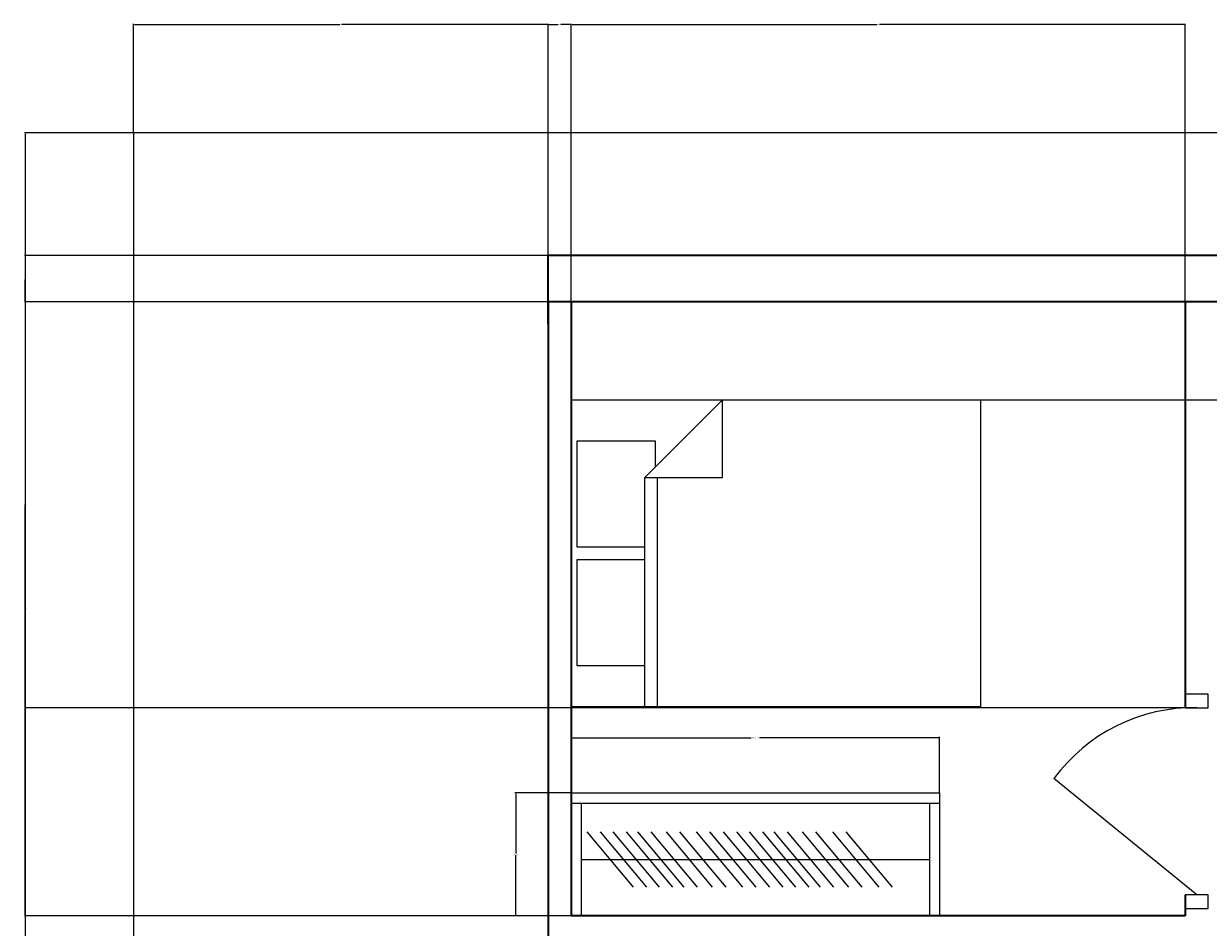
# Model space of a CAD drawing. Units: inches. Extents: x 109 to 572, y -157 to 568.
# Tile 2 of 5: x 109 to 341, y 391 to 568. Entities that reach past the tile are written whole.
import ezdxf

# ---------------------------------------------------------------- set-up
doc = ezdxf.new("R2010")
doc.units = ezdxf.units.IN
for name, color, linetype, lineweight in [('A-ANNO-DIMS', 2, 'Continuous', 18), ('A-FLOR-CASE', 32, 'Continuous', 18), ('A-WALL', 7, 'Continuous', 35), ('C-PROP', 8, 'Continuous', 18), ('DOOR.', 240, 'Continuous', 25), ('FURNUTURE', 50, 'Continuous', 18)]:
    doc.layers.add(name, color=color, linetype=linetype, lineweight=lineweight)
doc.styles.get("Standard").update_dxf_attribs({"font": 'arial.ttf'})
doc.dimstyles.get("Standard").update_dxf_attribs({"dimtxt": 0.18, "dimasz": 0.18, "dimexe": 0.18, "dimexo": 0.0625, "dimgap": 0.09, "dimtad": 0, "dimtih": 1, "dimtoh": 1, "dimdec": 4, "dimzin": 0, "dimdsep": 46, "dimtxsty": 'Standard', "dimcen": 0.09, "dimadec": 0, "dimazin": 0, "dimtfac": 1, "dimtdec": 4, "dimtofl": 0, "dimtmove": 0, "dimatfit": 3, "dimfxl": 1, "dimtolj": 1, "dimtzin": 0, "dimarcsym": 0})

# ---------------------------------------------------------------- blocks, each defined once
blk = doc.blocks.new('Bed - Queen')
for p, q in [((0, -80.00003), (0, 0)), ((0, 0), (59.99999, 0)), ((59.99999, 0), (59.99999, -80.00003)), ((7.99999, -1.2), (28.79998, -1.2)), ((7.99999, -14.4), (7.99999, -1.2)), ((28.79998, -1.2), (28.79998, -14.4)), ((31.19999, -1.2), (51.99999, -1.2)), ((31.19999, -14.4), (31.19999, -1.2)), ((51.99999, -1.2), (51.99999, -16.4)), ((0, -14.4), (44.8, -14.4)), ((59.99999, -29.6), (44.8, -14.4)), ((44.8, -14.4), (44.8, -29.6)), ((44.8, -16.8), (0, -16.8)), ((51.99999, -16.4), (46.79936, -16.4)), ((44.8, -29.6), (59.99999, -29.6)), ((59.99999, -80.00003), (0, -80.00003))]:
    blk.add_line(p, q)
blk = doc.blocks.new('DOOR-SINGLE-36IN-JAMB')
blk.add_line((0, 0), (-27.91, 22.73))
for points in [[(-2.25, 36.57), (2.25, 36.57), (2.25, 39.21), (-2.25, 39.21)], [(-2.25, -2.64), (2.25, -2.64), (2.25, 0), (-2.25, 0)]]:
    blk.add_lwpolyline(points, close=True)
blk.add_arc((-0.58, 2.67), 33.9, 89.0125, 143.7179)
blk = doc.blocks.new('CLOSET-FRAME-RAIL-72IN')
for p, q in [((0, 0), (0, 24)), ((0, 24), (72, 24)), ((72, 24), (72, 0)), ((0, 22), (72, 22)), ((2, 0), (2, 22)), ((70, 22), (70, 0)), ((2, 11), (70, 11))]:
    blk.add_line(p, q)
blk = doc.blocks.new('CLOSET-HANGERS')
for p, q in [((0, 0), (-9.05, 10.83)), ((2.61, -0.01), (-6.44, 10.82)), ((5.08, -0.01), (-3.97, 10.82)), ((7.69, -0.01), (-1.36, 10.82)), ((9.9, -0.01), (0.85, 10.82)), ((12.51, -0.01), (3.46, 10.82)), ((15.48, -0.01), (6.43, 10.82)), ((18.09, -0.01), (9.04, 10.82)), ((21.4, -0.01), (12.35, 10.82)), ((24.01, -0.01), (14.96, 10.82)), ((26.62, 0.01), (17.57, 10.84)), ((29.23, 0), (20.18, 10.83)), ((31.7, 0), (22.65, 10.83)), ((34.31, -0.01), (25.26, 10.82)), ((36.52, 0), (27.47, 10.83)), ((39.13, -0.01), (30.08, 10.82)), ((42.1, 0), (33.05, 10.83)), ((44.71, -0.01), (35.66, 10.82)), ((48.01, 0), (38.97, 10.83)), ((50.63, -0.01), (41.58, 10.82))]:
    blk.add_line(p, q)
blk = doc.blocks.new('*D25')
at = {"layer": 'A-ANNO-DIMS', "color": 0, "lineweight": -2, "transparency": 16777216}
for p, q in [((216.02, 417.6), (216.02, 428.52)), ((216.2, 428.34), (251.18, 428.34)), ((287.84, 428.34), (252.86, 428.34)), ((288.02, 417.6), (288.02, 428.52))]:
    blk.add_line(p, q, dxfattribs=at)
at = {"layer": 'A-ANNO-DIMS', "color": 0, "transparency": 16777216}
for points in [[(216.2, 428.37), (216.2, 428.31), (216.02, 428.34)], [(287.84, 428.37), (287.84, 428.31), (288.02, 428.34)]]:
    blk.add_solid(points, dxfattribs=at)
at = {"layer": 'Defpoints', "color": 0, "transparency": 16777216}
for p in [(288.02, 428.34), (216.02, 417.54), (288.02, 417.54)]:
    blk.add_point(p, dxfattribs=at)
at = {"layer": 'A-ANNO-DIMS', "color": 0, "transparency": 16777216, "insert": (252.02, 428.34), "char_height": 0.18, "attachment_point": 5}
blk.add_mtext('\\A1;RAIL 72 TYP.', dxfattribs=at)
blk = doc.blocks.new('*D26')
at = {"layer": 'A-ANNO-DIMS', "color": 0, "lineweight": -2, "transparency": 16777216}
for p, q in [((215.96, 417.54), (205.04, 417.54)), ((205.22, 417.36), (205.22, 405.72)), ((205.22, 393.72), (205.22, 405.36)), ((215.96, 393.54), (205.04, 393.54))]:
    blk.add_line(p, q, dxfattribs=at)
at = {"layer": 'A-ANNO-DIMS', "color": 0, "transparency": 16777216}
for points in [[(205.19, 417.36), (205.25, 417.36), (205.22, 417.54)], [(205.19, 393.72), (205.25, 393.72), (205.22, 393.54)]]:
    blk.add_solid(points, dxfattribs=at)
at = {"layer": 'Defpoints', "color": 0, "transparency": 16777216}
for p in [(205.22, 417.54), (216.02, 417.54), (216.02, 393.54)]:
    blk.add_point(p, dxfattribs=at)
at = {"layer": 'A-ANNO-DIMS', "color": 0, "transparency": 16777216, "insert": (205.22, 405.54), "char_height": 0.18, "attachment_point": 5}
blk.add_mtext('\\A1;24 TYP.', dxfattribs=at)
blk = doc.blocks.new('*D40')
at = {"layer": 'A-ANNO-DIMS', "color": 0, "lineweight": -2, "transparency": 16777216}
for p, q in [((130.46, 546.54), (109.19, 546.54)), ((109.37, 546.36), (109.37, 336.72)), ((109.37, 126.72), (109.37, 336.36)), ((130.46, 126.54), (109.19, 126.54))]:
    blk.add_line(p, q, dxfattribs=at)
at = {"layer": 'A-ANNO-DIMS', "color": 0, "transparency": 16777216}
for points in [[(109.34, 546.36), (109.4, 546.36), (109.37, 546.54)], [(109.34, 126.72), (109.4, 126.72), (109.37, 126.54)]]:
    blk.add_solid(points, dxfattribs=at)
at = {"layer": 'Defpoints', "color": 0, "transparency": 16777216}
for p in [(109.37, 546.54), (130.52, 546.54), (130.52, 126.54)]:
    blk.add_point(p, dxfattribs=at)
at = {"layer": 'A-ANNO-DIMS', "color": 0, "transparency": 16777216, "insert": (109.37, 336.54), "char_height": 0.18, "attachment_point": 5}
blk.add_mtext('\\A1;420', dxfattribs=at)
blk = doc.blocks.new('*D41')
at = {"layer": 'A-ANNO-DIMS', "color": 0, "lineweight": -2, "transparency": 16777216}
for p, q in [((130.52, 546.6), (130.52, 567.87)), ((130.7, 567.69), (170.82, 567.69)), ((211.34, 567.69), (171.22, 567.69)), ((211.52, 522.6), (211.52, 567.87))]:
    blk.add_line(p, q, dxfattribs=at)
at = {"layer": 'A-ANNO-DIMS', "color": 0, "transparency": 16777216}
for points in [[(130.7, 567.72), (130.7, 567.66), (130.52, 567.69)], [(211.34, 567.72), (211.34, 567.66), (211.52, 567.69)]]:
    blk.add_solid(points, dxfattribs=at)
at = {"layer": 'Defpoints', "color": 0, "transparency": 16777216}
for p in [(211.52, 567.69), (130.52, 546.54), (211.52, 522.54)]:
    blk.add_point(p, dxfattribs=at)
at = {"layer": 'A-ANNO-DIMS', "color": 0, "transparency": 16777216, "insert": (171.02, 567.69), "char_height": 0.18, "attachment_point": 5}
blk.add_mtext('\\A1;81', dxfattribs=at)
blk = doc.blocks.new('*D45')
at = {"layer": 'A-ANNO-DIMS', "color": 0, "lineweight": -2, "transparency": 16777216}
for p, q in [((216.02, 513.6), (216.02, 567.87)), ((216.2, 567.69), (275.74, 567.69)), ((335.84, 567.69), (276.3, 567.69)), ((336.02, 513.6), (336.02, 567.87))]:
    blk.add_line(p, q, dxfattribs=at)
at = {"layer": 'A-ANNO-DIMS', "color": 0, "transparency": 16777216}
for points in [[(216.2, 567.72), (216.2, 567.66), (216.02, 567.69)], [(335.84, 567.72), (335.84, 567.66), (336.02, 567.69)]]:
    blk.add_solid(points, dxfattribs=at)
at = {"layer": 'Defpoints', "color": 0, "transparency": 16777216}
for p in [(336.02, 567.69), (216.02, 513.54), (336.02, 513.54)]:
    blk.add_point(p, dxfattribs=at)
at = {"layer": 'A-ANNO-DIMS', "color": 0, "transparency": 16777216, "insert": (276.02, 567.69), "char_height": 0.18, "attachment_point": 5}
blk.add_mtext('\\A1;120', dxfattribs=at)
blk = doc.blocks.new('*D50')
at = {"layer": 'A-ANNO-DIMS', "color": 0, "lineweight": -2, "transparency": 16777216}
for p, q in [((215.96, 513.54), (109.19, 513.54)), ((109.37, 513.36), (109.37, 453.72)), ((109.37, 393.72), (109.37, 453.36)), ((215.96, 393.54), (109.19, 393.54))]:
    blk.add_line(p, q, dxfattribs=at)
at = {"layer": 'A-ANNO-DIMS', "color": 0, "transparency": 16777216}
for points in [[(109.34, 513.36), (109.4, 513.36), (109.37, 513.54)], [(109.34, 393.72), (109.4, 393.72), (109.37, 393.54)]]:
    blk.add_solid(points, dxfattribs=at)
at = {"layer": 'Defpoints', "color": 0, "transparency": 16777216}
for p in [(109.37, 513.54), (216.02, 513.54), (216.02, 393.54)]:
    blk.add_point(p, dxfattribs=at)
at = {"layer": 'A-ANNO-DIMS', "color": 0, "transparency": 16777216, "insert": (109.37, 453.54), "char_height": 0.18, "attachment_point": 5}
blk.add_mtext('\\A1;120', dxfattribs=at)
blk = doc.blocks.new('*D57')
at = {"layer": 'A-ANNO-DIMS', "color": 0, "lineweight": -2, "transparency": 16777216}
for p, q in [((335.96, 513.54), (109.19, 513.54)), ((109.37, 513.36), (109.37, 474.05)), ((109.37, 434.39), (109.37, 473.69)), ((335.96, 434.21), (109.19, 434.21))]:
    blk.add_line(p, q, dxfattribs=at)
at = {"layer": 'A-ANNO-DIMS', "color": 0, "transparency": 16777216}
for points in [[(109.34, 513.36), (109.4, 513.36), (109.37, 513.54)], [(109.34, 434.39), (109.4, 434.39), (109.37, 434.21)]]:
    blk.add_solid(points, dxfattribs=at)
at = {"layer": 'Defpoints', "color": 0, "transparency": 16777216}
for p in [(336.02, 513.54), (109.37, 434.21), (336.02, 434.21)]:
    blk.add_point(p, dxfattribs=at)
at = {"layer": 'A-ANNO-DIMS', "color": 0, "transparency": 16777216, "insert": (109.37, 473.87), "char_height": 0.18, "attachment_point": 5}
blk.add_mtext('\\A1;79.33', dxfattribs=at)
blk = doc.blocks.new('*D64')
at = {"layer": 'A-ANNO-DIMS', "color": 0, "lineweight": -2, "transparency": 16777216}
for p, q in [((211.52, 522.6), (211.52, 567.87)), ((211.7, 567.69), (213.51, 567.69)), ((215.84, 567.69), (214.03, 567.69)), ((216.02, 513.6), (216.02, 567.87))]:
    blk.add_line(p, q, dxfattribs=at)
at = {"layer": 'A-ANNO-DIMS', "color": 0, "transparency": 16777216}
for points in [[(211.7, 567.72), (211.7, 567.66), (211.52, 567.69)], [(215.84, 567.72), (215.84, 567.66), (216.02, 567.69)]]:
    blk.add_solid(points, dxfattribs=at)
at = {"layer": 'Defpoints', "color": 0, "transparency": 16777216}
for p in [(216.02, 567.69), (211.52, 522.54), (216.02, 513.54)]:
    blk.add_point(p, dxfattribs=at)
at = {"layer": 'A-ANNO-DIMS', "color": 0, "transparency": 16777216, "insert": (213.77, 567.69), "char_height": 0.18, "attachment_point": 5}
blk.add_mtext('\\A1;4.5', dxfattribs=at)
blk = doc.blocks.new('*D65')
at = {"layer": 'A-ANNO-DIMS', "color": 0, "lineweight": -2, "transparency": 16777216}
for p, q in [((211.46, 522.54), (109.19, 522.54)), ((109.37, 522.36), (109.37, 518.22)), ((109.37, 513.72), (109.37, 517.86)), ((215.96, 513.54), (109.19, 513.54))]:
    blk.add_line(p, q, dxfattribs=at)
at = {"layer": 'A-ANNO-DIMS', "color": 0, "transparency": 16777216}
for points in [[(109.34, 522.36), (109.4, 522.36), (109.37, 522.54)], [(109.34, 513.72), (109.4, 513.72), (109.37, 513.54)]]:
    blk.add_solid(points, dxfattribs=at)
at = {"layer": 'Defpoints', "color": 0, "transparency": 16777216}
for p in [(211.52, 522.54), (109.37, 513.54), (216.02, 513.54)]:
    blk.add_point(p, dxfattribs=at)
at = {"layer": 'A-ANNO-DIMS', "color": 0, "transparency": 16777216, "insert": (109.37, 518.04), "char_height": 0.18, "attachment_point": 5}
blk.add_mtext('\\A1;9', dxfattribs=at)
blk = doc.blocks.new('*D68')
at = {"layer": 'A-ANNO-DIMS', "color": 0, "lineweight": -2, "transparency": 16777216}
for p, q in [((216.08, 513.54), (571.85, 513.54)), ((571.67, 513.36), (571.67, 504.14)), ((571.67, 494.56), (571.67, 503.78)), ((216.08, 494.38), (571.85, 494.38))]:
    blk.add_line(p, q, dxfattribs=at)
at = {"layer": 'A-ANNO-DIMS', "color": 0, "transparency": 16777216}
for points in [[(571.64, 513.36), (571.7, 513.36), (571.67, 513.54)], [(571.64, 494.56), (571.7, 494.56), (571.67, 494.38)]]:
    blk.add_solid(points, dxfattribs=at)
at = {"layer": 'Defpoints', "color": 0, "transparency": 16777216}
for p in [(216.02, 513.54), (216.02, 494.38), (571.67, 494.38)]:
    blk.add_point(p, dxfattribs=at)
at = {"layer": 'A-ANNO-DIMS', "color": 0, "transparency": 16777216, "insert": (571.67, 503.96), "char_height": 0.18, "attachment_point": 5}
blk.add_mtext('\\A1;19.164', dxfattribs=at)

msp = doc.modelspace()

# ---------------------------------------------------------------- linework, layer by layer
at = {"layer": 'A-WALL'}
for p, q in [((526.5195, 522.5398), (211.5195, 522.5398)), ((211.5195, 509.301), (211.5195, 522.5398)), ((517.5195, 513.5398), (211.5195, 513.5398)), ((211.5195, 513.5398), (211.5195, 195.5398)), ((216.0195, 513.5398), (216.0195, 393.5398)), ((336.0195, 513.5398), (336.0195, 434.1697)), ((336.0195, 397.6358), (336.0195, 393.5398)), ((336.0195, 393.5398), (216.0195, 393.5398))]:
    msp.add_line(p, q, dxfattribs=at)
at = {"layer": 'C-PROP'}
for p, q in [((550.5195, 546.5398), (130.5195, 546.5398)), ((130.5195, 546.5398), (130.5195, 126.5398))]:
    msp.add_line(p, q, dxfattribs=at)

# ---------------------------------------------------------------- block references
at = {"layer": 'A-FLOR-CASE'}
for name, p in [('CLOSET-FRAME-RAIL-72IN', (216.0195, 393.5398)), ('CLOSET-HANGERS', (228.1956, 399.125))]:
    msp.add_blockref(name, p, dxfattribs=at)
at = {"layer": 'DOOR.'}
msp.add_blockref('DOOR-SINGLE-36IN-JAMB', (338.2695, 397.6358), dxfattribs=at)
at = {"layer": 'FURNUTURE', "rotation": 90}
msp.add_blockref('Bed - Queen', (216.0195, 434.3755), dxfattribs=at)

# ---------------------------------------------------------------- dimensions: what is measured, and where the dimension line sits
at = {"layer": 'A-ANNO-DIMS'}
for base, p1, p2, override, picture, middle in [((211.5195, 567.6898), (130.5195, 546.5398), (211.5195, 522.5398), {"dimdec": 0, "dimlfac": 1, "dimrnd": 0, "dimzin": 0, "dimdsep": 46, "dimlunit": 2}, '*D41', (171.0195, 567.6898)), ((216.0195, 567.6898), (211.5195, 522.5398), (216.0195, 513.5398), {"dimdec": 1, "dimlfac": 1, "dimrnd": 0, "dimzin": 0, "dimdsep": 46, "dimlunit": 2}, '*D64', (213.7695, 567.6898)), ((336.0195, 567.6898), (216.0195, 513.5398), (336.0195, 513.5398), {"dimdec": 0, "dimlfac": 1, "dimrnd": 0, "dimzin": 0, "dimdsep": 46, "dimlunit": 2}, '*D45', (276.0195, 567.6898))]:
    dim = msp.add_linear_dim(base=base, p1=p1, p2=p2, dimstyle='Standard', override=override, dxfattribs=at)
    dim.commit()
    dim.dimension.update_dxf_attribs({"geometry": picture, "text_midpoint": middle})
for base, p1, p2, override, picture, middle in [((109.3695, 546.5398), (130.5195, 126.5398), (130.5195, 546.5398), {"dimdec": 0, "dimlfac": 1, "dimrnd": 0, "dimzin": 0, "dimdsep": 46, "dimlunit": 2}, '*D40', (109.3695, 336.5398)), ((109.3695, 513.5398), (211.5195, 522.5398), (216.0195, 513.5398), {"dimdec": 0, "dimlfac": 1, "dimrnd": 0, "dimzin": 0, "dimdsep": 46, "dimlunit": 2}, '*D65', (109.3695, 518.0398)), ((109.3695, 434.2056), (336.0195, 513.5398), (336.0195, 434.2056), {"dimdec": 2, "dimlfac": 1, "dimrnd": 0, "dimzin": 0, "dimdsep": 46, "dimlunit": 2}, '*D57', (109.3695, 473.8727)), ((109.3695, 513.5398), (216.0195, 393.5398), (216.0195, 513.5398), {"dimdec": 0, "dimlfac": 1, "dimrnd": 0, "dimzin": 0, "dimdsep": 46, "dimlunit": 2}, '*D50', (109.3695, 453.5398)), ((571.6695, 494.3755), (216.0195, 513.5398), (216.0195, 494.3755), {"dimdec": 3, "dimlfac": 1, "dimrnd": 0, "dimzin": 0, "dimdsep": 46, "dimlunit": 2}, '*D68', (571.6695, 503.9576))]:
    dim = msp.add_linear_dim(base=base, p1=p1, p2=p2, angle=90, dimstyle='Standard', override=override, dxfattribs=at)
    dim.commit()
    dim.dimension.update_dxf_attribs({"geometry": picture, "text_midpoint": middle})
dim = msp.add_linear_dim(base=(288.0195, 428.3398), p1=(216.0195, 417.5398), p2=(288.0195, 417.5398), text='RAIL <> TYP.', dimstyle='Standard', override={"dimdec": 0, "dimlfac": 1, "dimrnd": 0, "dimzin": 0, "dimdsep": 46, "dimlunit": 2}, dxfattribs=at)
dim.commit()
dim.dimension.update_dxf_attribs({"geometry": '*D25', "text_midpoint": (252.0195, 428.3398)})
dim = msp.add_linear_dim(base=(205.2195, 417.5398), p1=(216.0195, 393.5398), p2=(216.0195, 417.5398), angle=90, text='<> TYP.', dimstyle='Standard', override={"dimdec": 0, "dimlfac": 1, "dimrnd": 0, "dimzin": 0, "dimdsep": 46, "dimlunit": 2}, dxfattribs=at)
dim.commit()
dim.dimension.update_dxf_attribs({"geometry": '*D26', "text_midpoint": (205.2195, 405.5398)})

doc.saveas('drawing.dxf')
